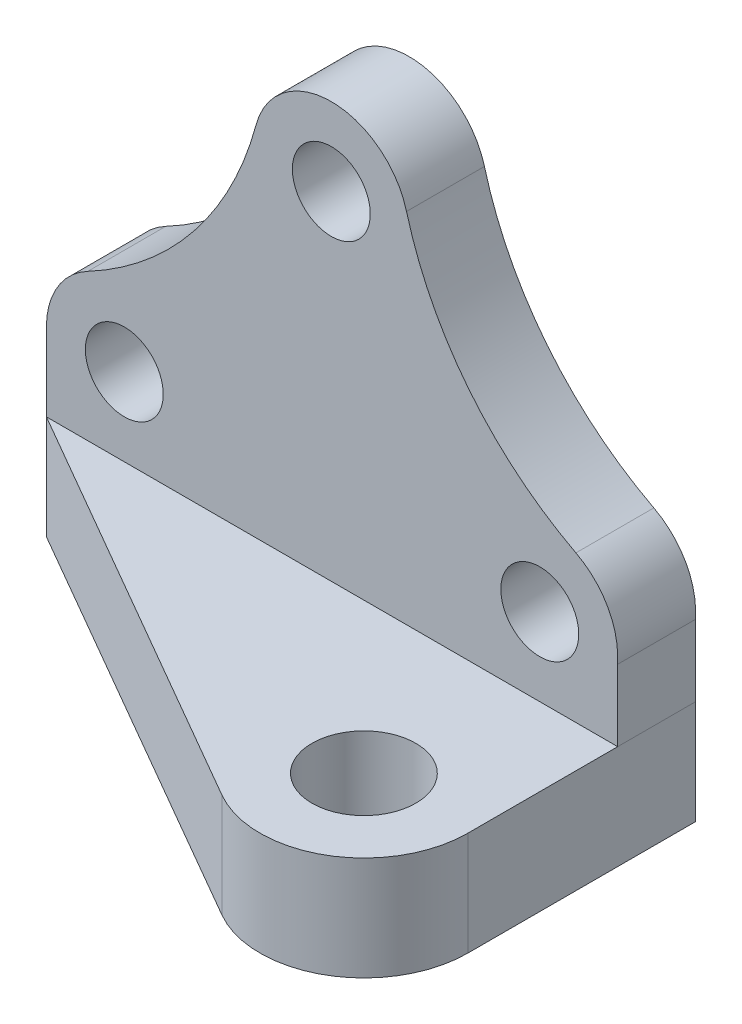
ISO-10303-21;
HEADER;
FILE_DESCRIPTION(('STEP AP214'),'2;1');
FILE_NAME('part.step','',(''),(''),'','','');
FILE_SCHEMA(('AUTOMOTIVE_DESIGN { 1 0 10303 214 1 1 1 1 }'));
ENDSEC;
DATA;
#1=APPLICATION_CONTEXT('core data for automotive mechanical design processes');
#2=APPLICATION_PROTOCOL_DEFINITION('international standard','automotive_design',2000,#1);
#3=PRODUCT_CONTEXT('',#1,'mechanical');
#4=PRODUCT('Part','Part','',(#3));
#5=PRODUCT_RELATED_PRODUCT_CATEGORY('part','',(#4));
#6=PRODUCT_DEFINITION_FORMATION('','',#4);
#7=PRODUCT_DEFINITION_CONTEXT('part definition',#1,'design');
#8=PRODUCT_DEFINITION('design','',#6,#7);
#9=PRODUCT_DEFINITION_SHAPE('','',#8);
#10=(LENGTH_UNIT() NAMED_UNIT(*) SI_UNIT(.MILLI.,.METRE.));
#11=(NAMED_UNIT(*) PLANE_ANGLE_UNIT() SI_UNIT($,.RADIAN.));
#12=(NAMED_UNIT(*) SI_UNIT($,.STERADIAN.) SOLID_ANGLE_UNIT());
#13=UNCERTAINTY_MEASURE_WITH_UNIT(LENGTH_MEASURE(1.E-05),#10,'distance_accuracy_value','');
#14=(GEOMETRIC_REPRESENTATION_CONTEXT(3) GLOBAL_UNCERTAINTY_ASSIGNED_CONTEXT((#13)) GLOBAL_UNIT_ASSIGNED_CONTEXT((#10,
#11,#12)) REPRESENTATION_CONTEXT('',''));
#15=CARTESIAN_POINT('',(0.,0.,0.));
#16=DIRECTION('',(0.,0.,1.));
#17=DIRECTION('',(1.,0.,0.));
#18=AXIS2_PLACEMENT_3D('',#15,#16,#17);
#19=CARTESIAN_POINT('',(0.,-20.,0.));
#20=DIRECTION('',(-0.500000000000001,0.,0.866025403784438));
#21=DIRECTION('',(0.866025403784438,0.,0.500000000000001));
#22=AXIS2_PLACEMENT_3D('',#19,#20,#21);
#23=PLANE('',#22);
#24=DIRECTION('',(0.866025403784438,0.,0.500000000000001));
#25=VECTOR('',#24,1.);
#26=CARTESIAN_POINT('',(0.,0.,0.));
#27=LINE('',#26,#25);
#28=CARTESIAN_POINT('',(0.,0.,0.));
#29=VERTEX_POINT('',#28);
#30=CARTESIAN_POINT('',(80.,0.,46.1880215351702));
#31=VERTEX_POINT('',#30);
#32=EDGE_CURVE('E102',#29,#31,#27,.T.);
#33=ORIENTED_EDGE('',*,*,#32,.F.);
#34=DIRECTION('',(0.,1.,0.));
#35=VECTOR('',#34,1.);
#36=CARTESIAN_POINT('',(0.,-20.,0.));
#37=LINE('',#36,#35);
#38=CARTESIAN_POINT('',(0.,-20.,0.));
#39=VERTEX_POINT('',#38);
#40=EDGE_CURVE('E11',#39,#29,#37,.T.);
#41=ORIENTED_EDGE('',*,*,#40,.F.);
#42=DIRECTION('',(0.866025403784438,0.,0.500000000000001));
#43=VECTOR('',#42,1.);
#44=CARTESIAN_POINT('',(0.,-20.,0.));
#45=LINE('',#44,#43);
#46=CARTESIAN_POINT('',(80.,-20.,46.1880215351702));
#47=VERTEX_POINT('',#46);
#48=EDGE_CURVE('E114',#39,#47,#45,.T.);
#49=ORIENTED_EDGE('',*,*,#48,.T.);
#50=DIRECTION('',(0.,1.,0.));
#51=VECTOR('',#50,1.);
#52=CARTESIAN_POINT('',(80.,-20.,46.1880215351702));
#53=LINE('',#52,#51);
#54=EDGE_CURVE('E42',#47,#31,#53,.T.);
#55=ORIENTED_EDGE('',*,*,#54,.T.);
#56=EDGE_LOOP('',(#33,#41,#49,#55));
#57=FACE_BOUND('',#56,.T.);
#58=ADVANCED_FACE('F41',(#57),#23,.T.);
#59=CARTESIAN_POINT('',(110.,-20.,0.));
#60=DIRECTION('',(1.,0.,0.));
#61=DIRECTION('',(0.,0.,-1.));
#62=AXIS2_PLACEMENT_3D('',#59,#60,#61);
#63=PLANE('',#62);
#64=DIRECTION('',(0.,0.,-1.));
#65=VECTOR('',#64,1.);
#66=CARTESIAN_POINT('',(110.,0.,0.));
#67=LINE('',#66,#65);
#68=CARTESIAN_POINT('',(110.,0.,28.8675134594814));
#69=VERTEX_POINT('',#68);
#70=CARTESIAN_POINT('',(110.,0.,0.));
#71=VERTEX_POINT('',#70);
#72=EDGE_CURVE('E115',#69,#71,#67,.T.);
#73=ORIENTED_EDGE('',*,*,#72,.F.);
#74=DIRECTION('',(0.,1.,0.));
#75=VECTOR('',#74,1.);
#76=CARTESIAN_POINT('',(110.,-20.,28.8675134594814));
#77=LINE('',#76,#75);
#78=CARTESIAN_POINT('',(110.,-20.,28.8675134594814));
#79=VERTEX_POINT('',#78);
#80=EDGE_CURVE('E49',#79,#69,#77,.T.);
#81=ORIENTED_EDGE('',*,*,#80,.F.);
#82=DIRECTION('',(0.,0.,-1.));
#83=VECTOR('',#82,1.);
#84=CARTESIAN_POINT('',(110.,-20.,0.));
#85=LINE('',#84,#83);
#86=CARTESIAN_POINT('',(110.,-20.,-15.));
#87=VERTEX_POINT('',#86);
#88=EDGE_CURVE('E118',#79,#87,#85,.T.);
#89=ORIENTED_EDGE('',*,*,#88,.T.);
#90=DIRECTION('',(0.,-1.,0.));
#91=VECTOR('',#90,1.);
#92=CARTESIAN_POINT('',(110.,0.,-15.));
#93=LINE('',#92,#91);
#94=CARTESIAN_POINT('',(110.,0.,-15.));
#95=VERTEX_POINT('',#94);
#96=EDGE_CURVE('E138',#95,#87,#93,.T.);
#97=ORIENTED_EDGE('',*,*,#96,.F.);
#98=DIRECTION('',(0.,0.,1.));
#99=VECTOR('',#98,1.);
#100=CARTESIAN_POINT('',(110.,0.,-15.));
#101=LINE('',#100,#99);
#102=EDGE_CURVE('E186',#95,#71,#101,.T.);
#103=ORIENTED_EDGE('',*,*,#102,.T.);
#104=EDGE_LOOP('',(#73,#81,#89,#97,#103));
#105=FACE_BOUND('',#104,.T.);
#106=ADVANCED_FACE('F224',(#105),#63,.T.);
#107=CARTESIAN_POINT('',(90.,-20.,28.8675134594814));
#108=DIRECTION('',(0.,1.,0.));
#109=DIRECTION('',(0.,0.,1.));
#110=AXIS2_PLACEMENT_3D('',#107,#108,#109);
#111=CYLINDRICAL_SURFACE('',#110,20.);
#112=CARTESIAN_POINT('',(90.,0.,28.8675134594814));
#113=DIRECTION('',(0.,1.,0.));
#114=DIRECTION('',(0.,0.,1.));
#115=AXIS2_PLACEMENT_3D('',#112,#113,#114);
#116=CIRCLE('',#115,20.);
#117=EDGE_CURVE('E110',#31,#69,#116,.T.);
#118=ORIENTED_EDGE('',*,*,#117,.F.);
#119=ORIENTED_EDGE('',*,*,#54,.F.);
#120=CARTESIAN_POINT('',(90.,-20.,28.8675134594814));
#121=DIRECTION('',(0.,1.,0.));
#122=DIRECTION('',(0.,0.,1.));
#123=AXIS2_PLACEMENT_3D('',#120,#121,#122);
#124=CIRCLE('',#123,20.);
#125=EDGE_CURVE('E113',#47,#79,#124,.T.);
#126=ORIENTED_EDGE('',*,*,#125,.T.);
#127=ORIENTED_EDGE('',*,*,#80,.T.);
#128=EDGE_LOOP('',(#118,#119,#126,#127));
#129=FACE_BOUND('',#128,.T.);
#130=ADVANCED_FACE('F124',(#129),#111,.T.);
#131=CARTESIAN_POINT('',(90.,-20.,28.8675134594814));
#132=DIRECTION('',(0.,1.,0.));
#133=DIRECTION('',(0.,0.,1.));
#134=AXIS2_PLACEMENT_3D('',#131,#132,#133);
#135=PLANE('',#134);
#136=CARTESIAN_POINT('',(90.,-20.,28.8675134594814));
#137=DIRECTION('',(0.,1.,0.));
#138=DIRECTION('',(0.,0.,1.));
#139=AXIS2_PLACEMENT_3D('',#136,#137,#138);
#140=CIRCLE('',#139,9.99999999999999);
#141=CARTESIAN_POINT('',(90.,-20.,38.8675134594814));
#142=VERTEX_POINT('',#141);
#143=EDGE_CURVE('E107',#142,#142,#140,.T.);
#144=ORIENTED_EDGE('',*,*,#143,.T.);
#145=EDGE_LOOP('',(#144));
#146=FACE_BOUND('',#145,.T.);
#147=ORIENTED_EDGE('',*,*,#48,.F.);
#148=DIRECTION('',(0.,0.,1.));
#149=VECTOR('',#148,1.);
#150=CARTESIAN_POINT('',(0.,-20.,-15.));
#151=LINE('',#150,#149);
#152=CARTESIAN_POINT('',(0.,-20.,-15.));
#153=VERTEX_POINT('',#152);
#154=EDGE_CURVE('E97',#153,#39,#151,.T.);
#155=ORIENTED_EDGE('',*,*,#154,.F.);
#156=DIRECTION('',(-1.,0.,0.));
#157=VECTOR('',#156,1.);
#158=CARTESIAN_POINT('',(0.,-20.,-15.));
#159=LINE('',#158,#157);
#160=EDGE_CURVE('E134',#87,#153,#159,.T.);
#161=ORIENTED_EDGE('',*,*,#160,.F.);
#162=ORIENTED_EDGE('',*,*,#88,.F.);
#163=ORIENTED_EDGE('',*,*,#125,.F.);
#164=EDGE_LOOP('',(#147,#155,#161,#162,#163));
#165=FACE_BOUND('',#164,.T.);
#166=ADVANCED_FACE('F126',(#146,#165),#135,.F.);
#167=CARTESIAN_POINT('',(90.,0.,28.8675134594814));
#168=DIRECTION('',(0.,1.,0.));
#169=DIRECTION('',(0.,0.,1.));
#170=AXIS2_PLACEMENT_3D('',#167,#168,#169);
#171=PLANE('',#170);
#172=CARTESIAN_POINT('',(90.,0.,28.8675134594814));
#173=DIRECTION('',(0.,1.,0.));
#174=DIRECTION('',(0.,0.,1.));
#175=AXIS2_PLACEMENT_3D('',#172,#173,#174);
#176=CIRCLE('',#175,9.99999999999999);
#177=CARTESIAN_POINT('',(90.,0.,38.8675134594814));
#178=VERTEX_POINT('',#177);
#179=EDGE_CURVE('E203',#178,#178,#176,.T.);
#180=ORIENTED_EDGE('',*,*,#179,.F.);
#181=EDGE_LOOP('',(#180));
#182=FACE_BOUND('',#181,.T.);
#183=ORIENTED_EDGE('',*,*,#32,.T.);
#184=ORIENTED_EDGE('',*,*,#117,.T.);
#185=ORIENTED_EDGE('',*,*,#72,.T.);
#186=DIRECTION('',(-1.,0.,0.));
#187=VECTOR('',#186,1.);
#188=CARTESIAN_POINT('',(0.,0.,0.));
#189=LINE('',#188,#187);
#190=EDGE_CURVE('E85',#71,#29,#189,.T.);
#191=ORIENTED_EDGE('',*,*,#190,.T.);
#192=EDGE_LOOP('',(#183,#184,#185,#191));
#193=FACE_BOUND('',#192,.T.);
#194=ADVANCED_FACE('F112',(#182,#193),#171,.T.);
#195=CARTESIAN_POINT('',(90.,-20.,28.8675134594814));
#196=DIRECTION('',(0.,1.,0.));
#197=DIRECTION('',(0.,0.,1.));
#198=AXIS2_PLACEMENT_3D('',#195,#196,#197);
#199=CYLINDRICAL_SURFACE('',#198,9.99999999999999);
#200=ORIENTED_EDGE('',*,*,#143,.F.);
#201=EDGE_LOOP('',(#200));
#202=FACE_BOUND('',#201,.T.);
#203=ORIENTED_EDGE('',*,*,#179,.T.);
#204=EDGE_LOOP('',(#203));
#205=FACE_BOUND('',#204,.T.);
#206=ADVANCED_FACE('F210',(#202,#205),#199,.F.);
#207=CARTESIAN_POINT('',(-22.4100448127981,85.7141325839781,-15.));
#208=DIRECTION('',(0.,0.,1.));
#209=DIRECTION('',(1.,0.,0.));
#210=AXIS2_PLACEMENT_3D('',#207,#208,#209);
#211=CYLINDRICAL_SURFACE('',#210,65.);
#212=CARTESIAN_POINT('',(-22.4100448127981,85.7141325839781,0.));
#213=DIRECTION('',(0.,0.,-1.));
#214=DIRECTION('',(-1.,0.,0.));
#215=AXIS2_PLACEMENT_3D('',#212,#213,#214);
#216=CIRCLE('',#215,65.);
#217=CARTESIAN_POINT('',(40.3732592292779,68.8838998594959,0.));
#218=VERTEX_POINT('',#217);
#219=CARTESIAN_POINT('',(7.98561659760035,28.2588998594959,0.));
#220=VERTEX_POINT('',#219);
#221=EDGE_CURVE('E158',#218,#220,#216,.T.);
#222=ORIENTED_EDGE('',*,*,#221,.F.);
#223=DIRECTION('',(0.,0.,1.));
#224=VECTOR('',#223,1.);
#225=CARTESIAN_POINT('',(40.3732592292779,68.8838998594959,-15.));
#226=LINE('',#225,#224);
#227=CARTESIAN_POINT('',(40.3732592292779,68.8838998594959,-15.));
#228=VERTEX_POINT('',#227);
#229=EDGE_CURVE('E196',#228,#218,#226,.T.);
#230=ORIENTED_EDGE('',*,*,#229,.F.);
#231=CARTESIAN_POINT('',(-22.4100448127981,85.7141325839781,-15.));
#232=DIRECTION('',(0.,0.,-1.));
#233=DIRECTION('',(-1.,0.,0.));
#234=AXIS2_PLACEMENT_3D('',#231,#232,#233);
#235=CIRCLE('',#234,65.);
#236=CARTESIAN_POINT('',(7.98561659760035,28.2588998594959,-15.));
#237=VERTEX_POINT('',#236);
#238=EDGE_CURVE('E179',#228,#237,#235,.T.);
#239=ORIENTED_EDGE('',*,*,#238,.T.);
#240=DIRECTION('',(0.,0.,1.));
#241=VECTOR('',#240,1.);
#242=CARTESIAN_POINT('',(7.98561659760035,28.2588998594959,-15.));
#243=LINE('',#242,#241);
#244=EDGE_CURVE('E160',#237,#220,#243,.T.);
#245=ORIENTED_EDGE('',*,*,#244,.T.);
#246=EDGE_LOOP('',(#222,#230,#239,#245));
#247=FACE_BOUND('',#246,.T.);
#248=ADVANCED_FACE('F216',(#247),#211,.F.);
#249=CARTESIAN_POINT('',(54.8617140082186,65.,-15.));
#250=DIRECTION('',(0.,0.,1.));
#251=DIRECTION('',(1.,0.,0.));
#252=AXIS2_PLACEMENT_3D('',#249,#250,#251);
#253=CYLINDRICAL_SURFACE('',#252,15.);
#254=CARTESIAN_POINT('',(54.8617140082186,65.,0.));
#255=DIRECTION('',(0.,0.,-1.));
#256=DIRECTION('',(-1.,0.,0.));
#257=AXIS2_PLACEMENT_3D('',#254,#255,#256);
#258=CIRCLE('',#257,15.);
#259=CARTESIAN_POINT('',(69.3416105706828,68.9156858326908,0.));
#260=VERTEX_POINT('',#259);
#261=EDGE_CURVE('E159',#218,#260,#258,.T.);
#262=ORIENTED_EDGE('',*,*,#261,.T.);
#263=DIRECTION('',(0.,0.,1.));
#264=VECTOR('',#263,1.);
#265=CARTESIAN_POINT('',(69.3416105706828,68.9156858326908,-15.));
#266=LINE('',#265,#264);
#267=CARTESIAN_POINT('',(69.3416105706828,68.9156858326908,-15.));
#268=VERTEX_POINT('',#267);
#269=EDGE_CURVE('E194',#268,#260,#266,.T.);
#270=ORIENTED_EDGE('',*,*,#269,.F.);
#271=CARTESIAN_POINT('',(54.8617140082186,65.,-15.));
#272=DIRECTION('',(0.,0.,-1.));
#273=DIRECTION('',(-1.,0.,0.));
#274=AXIS2_PLACEMENT_3D('',#271,#272,#273);
#275=CIRCLE('',#274,15.);
#276=EDGE_CURVE('E333',#228,#268,#275,.T.);
#277=ORIENTED_EDGE('',*,*,#276,.F.);
#278=ORIENTED_EDGE('',*,*,#229,.T.);
#279=EDGE_LOOP('',(#262,#270,#277,#278));
#280=FACE_BOUND('',#279,.T.);
#281=ADVANCED_FACE('F284',(#280),#253,.T.);
#282=CARTESIAN_POINT('',(132.087829008028,85.8836577743507,-15.));
#283=DIRECTION('',(0.,0.,1.));
#284=DIRECTION('',(1.,0.,0.));
#285=AXIS2_PLACEMENT_3D('',#282,#283,#284);
#286=CYLINDRICAL_SURFACE('',#285,65.);
#287=CARTESIAN_POINT('',(132.087829008028,85.8836577743507,0.));
#288=DIRECTION('',(0.,0.,-1.));
#289=DIRECTION('',(-1.,0.,0.));
#290=AXIS2_PLACEMENT_3D('',#287,#288,#289);
#291=CIRCLE('',#290,65.);
#292=CARTESIAN_POINT('',(101.953967939005,28.2906858326908,0.));
#293=VERTEX_POINT('',#292);
#294=EDGE_CURVE('E162',#293,#260,#291,.T.);
#295=ORIENTED_EDGE('',*,*,#294,.F.);
#296=DIRECTION('',(0.,0.,1.));
#297=VECTOR('',#296,1.);
#298=CARTESIAN_POINT('',(101.953967939005,28.2906858326908,-15.));
#299=LINE('',#298,#297);
#300=CARTESIAN_POINT('',(101.953967939005,28.2906858326908,-15.));
#301=VERTEX_POINT('',#300);
#302=EDGE_CURVE('E195',#301,#293,#299,.T.);
#303=ORIENTED_EDGE('',*,*,#302,.F.);
#304=CARTESIAN_POINT('',(132.087829008028,85.8836577743507,-15.));
#305=DIRECTION('',(0.,0.,-1.));
#306=DIRECTION('',(-1.,0.,0.));
#307=AXIS2_PLACEMENT_3D('',#304,#305,#306);
#308=CIRCLE('',#307,65.);
#309=EDGE_CURVE('E279',#301,#268,#308,.T.);
#310=ORIENTED_EDGE('',*,*,#309,.T.);
#311=ORIENTED_EDGE('',*,*,#269,.T.);
#312=EDGE_LOOP('',(#295,#303,#310,#311));
#313=FACE_BOUND('',#312,.T.);
#314=ADVANCED_FACE('F277',(#313),#286,.F.);
#315=CARTESIAN_POINT('',(95.,15.,-15.));
#316=DIRECTION('',(0.,0.,1.));
#317=DIRECTION('',(1.,0.,0.));
#318=AXIS2_PLACEMENT_3D('',#315,#316,#317);
#319=CYLINDRICAL_SURFACE('',#318,15.);
#320=CARTESIAN_POINT('',(95.,15.,0.));
#321=DIRECTION('',(0.,0.,-1.));
#322=DIRECTION('',(-1.,0.,0.));
#323=AXIS2_PLACEMENT_3D('',#320,#321,#322);
#324=CIRCLE('',#323,15.);
#325=CARTESIAN_POINT('',(109.941701745293,13.6788077525573,0.));
#326=VERTEX_POINT('',#325);
#327=EDGE_CURVE('E167',#293,#326,#324,.T.);
#328=ORIENTED_EDGE('',*,*,#327,.T.);
#329=DIRECTION('',(0.,0.,1.));
#330=VECTOR('',#329,1.);
#331=CARTESIAN_POINT('',(109.941701745293,13.6788077525573,-15.));
#332=LINE('',#331,#330);
#333=CARTESIAN_POINT('',(109.941701745293,13.6788077525573,-15.));
#334=VERTEX_POINT('',#333);
#335=EDGE_CURVE('E188',#334,#326,#332,.T.);
#336=ORIENTED_EDGE('',*,*,#335,.F.);
#337=CARTESIAN_POINT('',(95.,15.,-15.));
#338=DIRECTION('',(0.,0.,-1.));
#339=DIRECTION('',(-1.,0.,0.));
#340=AXIS2_PLACEMENT_3D('',#337,#338,#339);
#341=CIRCLE('',#340,15.);
#342=EDGE_CURVE('E341',#301,#334,#341,.T.);
#343=ORIENTED_EDGE('',*,*,#342,.F.);
#344=ORIENTED_EDGE('',*,*,#302,.T.);
#345=EDGE_LOOP('',(#328,#336,#343,#344));
#346=FACE_BOUND('',#345,.T.);
#347=ADVANCED_FACE('F289',(#346),#319,.T.);
#348=CARTESIAN_POINT('',(109.99800198193,0.468804858784846,-15.));
#349=DIRECTION('',(0.999990918058441,0.00426190105892585,0.));
#350=DIRECTION('',(-0.00426190105892585,0.999990918058441,0.));
#351=AXIS2_PLACEMENT_3D('',#348,#349,#350);
#352=PLANE('',#351);
#353=DIRECTION('',(-0.00426190105892585,0.999990918058441,0.));
#354=VECTOR('',#353,1.);
#355=CARTESIAN_POINT('',(109.99800198193,0.468804858784846,0.));
#356=LINE('',#355,#354);
#357=EDGE_CURVE('E89',#71,#326,#356,.T.);
#358=ORIENTED_EDGE('',*,*,#357,.F.);
#359=ORIENTED_EDGE('',*,*,#102,.F.);
#360=DIRECTION('',(-0.00426190105892585,0.999990918058441,0.));
#361=VECTOR('',#360,1.);
#362=CARTESIAN_POINT('',(109.99800198193,0.468804858784846,-15.));
#363=LINE('',#362,#361);
#364=EDGE_CURVE('E142',#95,#334,#363,.T.);
#365=ORIENTED_EDGE('',*,*,#364,.T.);
#366=ORIENTED_EDGE('',*,*,#335,.T.);
#367=EDGE_LOOP('',(#358,#359,#365,#366));
#368=FACE_BOUND('',#367,.T.);
#369=ADVANCED_FACE('F240',(#368),#352,.T.);
#370=CARTESIAN_POINT('',(0.,0.,-15.));
#371=DIRECTION('',(-1.,0.,0.));
#372=DIRECTION('',(0.,0.,1.));
#373=AXIS2_PLACEMENT_3D('',#370,#371,#372);
#374=PLANE('',#373);
#375=DIRECTION('',(0.,-1.,0.));
#376=VECTOR('',#375,1.);
#377=CARTESIAN_POINT('',(0.,0.,0.));
#378=LINE('',#377,#376);
#379=CARTESIAN_POINT('',(0.,15.,0.));
#380=VERTEX_POINT('',#379);
#381=EDGE_CURVE('E79',#380,#29,#378,.T.);
#382=ORIENTED_EDGE('',*,*,#381,.F.);
#383=DIRECTION('',(0.,0.,1.));
#384=VECTOR('',#383,1.);
#385=CARTESIAN_POINT('',(0.,15.,-15.));
#386=LINE('',#385,#384);
#387=CARTESIAN_POINT('',(0.,15.,-15.));
#388=VERTEX_POINT('',#387);
#389=EDGE_CURVE('E181',#388,#380,#386,.T.);
#390=ORIENTED_EDGE('',*,*,#389,.F.);
#391=DIRECTION('',(0.,-1.,0.));
#392=VECTOR('',#391,1.);
#393=CARTESIAN_POINT('',(0.,0.,-15.));
#394=LINE('',#393,#392);
#395=EDGE_CURVE('E140',#388,#153,#394,.T.);
#396=ORIENTED_EDGE('',*,*,#395,.T.);
#397=ORIENTED_EDGE('',*,*,#154,.T.);
#398=ORIENTED_EDGE('',*,*,#40,.T.);
#399=EDGE_LOOP('',(#382,#390,#396,#397,#398));
#400=FACE_BOUND('',#399,.T.);
#401=ADVANCED_FACE('F92',(#400),#374,.T.);
#402=CARTESIAN_POINT('',(15.,15.,-15.));
#403=DIRECTION('',(0.,0.,1.));
#404=DIRECTION('',(1.,0.,0.));
#405=AXIS2_PLACEMENT_3D('',#402,#403,#404);
#406=CYLINDRICAL_SURFACE('',#405,7.5);
#407=CARTESIAN_POINT('',(15.,15.,-15.));
#408=DIRECTION('',(0.,0.,-1.));
#409=DIRECTION('',(-1.,0.,0.));
#410=AXIS2_PLACEMENT_3D('',#407,#408,#409);
#411=CIRCLE('',#410,7.5);
#412=CARTESIAN_POINT('',(7.5,15.,-15.));
#413=VERTEX_POINT('',#412);
#414=EDGE_CURVE('E151',#413,#413,#411,.T.);
#415=ORIENTED_EDGE('',*,*,#414,.T.);
#416=EDGE_LOOP('',(#415));
#417=FACE_BOUND('',#416,.T.);
#418=CARTESIAN_POINT('',(15.,15.,0.));
#419=DIRECTION('',(0.,0.,-1.));
#420=DIRECTION('',(-1.,0.,0.));
#421=AXIS2_PLACEMENT_3D('',#418,#419,#420);
#422=CIRCLE('',#421,7.5);
#423=CARTESIAN_POINT('',(7.5,15.,0.));
#424=VERTEX_POINT('',#423);
#425=EDGE_CURVE('E173',#424,#424,#422,.T.);
#426=ORIENTED_EDGE('',*,*,#425,.F.);
#427=EDGE_LOOP('',(#426));
#428=FACE_BOUND('',#427,.T.);
#429=ADVANCED_FACE('F300',(#417,#428),#406,.F.);
#430=CARTESIAN_POINT('',(54.8617140082186,65.,-15.));
#431=DIRECTION('',(0.,0.,1.));
#432=DIRECTION('',(1.,0.,0.));
#433=AXIS2_PLACEMENT_3D('',#430,#431,#432);
#434=CYLINDRICAL_SURFACE('',#433,7.5);
#435=CARTESIAN_POINT('',(54.8617140082186,65.,-15.));
#436=DIRECTION('',(0.,0.,-1.));
#437=DIRECTION('',(-1.,0.,0.));
#438=AXIS2_PLACEMENT_3D('',#435,#436,#437);
#439=CIRCLE('',#438,7.5);
#440=CARTESIAN_POINT('',(47.3617140082186,65.,-15.));
#441=VERTEX_POINT('',#440);
#442=EDGE_CURVE('E146',#441,#441,#439,.T.);
#443=ORIENTED_EDGE('',*,*,#442,.T.);
#444=EDGE_LOOP('',(#443));
#445=FACE_BOUND('',#444,.T.);
#446=CARTESIAN_POINT('',(54.8617140082186,65.,0.));
#447=DIRECTION('',(0.,0.,-1.));
#448=DIRECTION('',(-1.,0.,0.));
#449=AXIS2_PLACEMENT_3D('',#446,#447,#448);
#450=CIRCLE('',#449,7.5);
#451=CARTESIAN_POINT('',(47.3617140082186,65.,0.));
#452=VERTEX_POINT('',#451);
#453=EDGE_CURVE('E174',#452,#452,#450,.T.);
#454=ORIENTED_EDGE('',*,*,#453,.F.);
#455=EDGE_LOOP('',(#454));
#456=FACE_BOUND('',#455,.T.);
#457=ADVANCED_FACE('F303',(#445,#456),#434,.F.);
#458=CARTESIAN_POINT('',(15.,15.,-15.));
#459=DIRECTION('',(0.,0.,1.));
#460=DIRECTION('',(1.,0.,0.));
#461=AXIS2_PLACEMENT_3D('',#458,#459,#460);
#462=CYLINDRICAL_SURFACE('',#461,15.);
#463=CARTESIAN_POINT('',(15.,15.,0.));
#464=DIRECTION('',(0.,0.,-1.));
#465=DIRECTION('',(-1.,0.,0.));
#466=AXIS2_PLACEMENT_3D('',#463,#464,#465);
#467=CIRCLE('',#466,15.);
#468=EDGE_CURVE('E87',#380,#220,#467,.T.);
#469=ORIENTED_EDGE('',*,*,#468,.T.);
#470=ORIENTED_EDGE('',*,*,#244,.F.);
#471=CARTESIAN_POINT('',(15.,15.,-15.));
#472=DIRECTION('',(0.,0.,-1.));
#473=DIRECTION('',(-1.,0.,0.));
#474=AXIS2_PLACEMENT_3D('',#471,#472,#473);
#475=CIRCLE('',#474,15.);
#476=EDGE_CURVE('E139',#388,#237,#475,.T.);
#477=ORIENTED_EDGE('',*,*,#476,.F.);
#478=ORIENTED_EDGE('',*,*,#389,.T.);
#479=EDGE_LOOP('',(#469,#470,#477,#478));
#480=FACE_BOUND('',#479,.T.);
#481=ADVANCED_FACE('F298',(#480),#462,.T.);
#482=CARTESIAN_POINT('',(95.,15.,-15.));
#483=DIRECTION('',(0.,0.,1.));
#484=DIRECTION('',(1.,0.,0.));
#485=AXIS2_PLACEMENT_3D('',#482,#483,#484);
#486=CYLINDRICAL_SURFACE('',#485,7.50000000000001);
#487=CARTESIAN_POINT('',(95.,15.,-15.));
#488=DIRECTION('',(0.,0.,-1.));
#489=DIRECTION('',(-1.,0.,0.));
#490=AXIS2_PLACEMENT_3D('',#487,#488,#489);
#491=CIRCLE('',#490,7.50000000000001);
#492=CARTESIAN_POINT('',(87.5,15.,-15.));
#493=VERTEX_POINT('',#492);
#494=EDGE_CURVE('E152',#493,#493,#491,.T.);
#495=ORIENTED_EDGE('',*,*,#494,.T.);
#496=EDGE_LOOP('',(#495));
#497=FACE_BOUND('',#496,.T.);
#498=CARTESIAN_POINT('',(95.,15.,0.));
#499=DIRECTION('',(0.,0.,-1.));
#500=DIRECTION('',(-1.,0.,0.));
#501=AXIS2_PLACEMENT_3D('',#498,#499,#500);
#502=CIRCLE('',#501,7.50000000000001);
#503=CARTESIAN_POINT('',(87.5,15.,0.));
#504=VERTEX_POINT('',#503);
#505=EDGE_CURVE('E180',#504,#504,#502,.T.);
#506=ORIENTED_EDGE('',*,*,#505,.F.);
#507=EDGE_LOOP('',(#506));
#508=FACE_BOUND('',#507,.T.);
#509=ADVANCED_FACE('F305',(#497,#508),#486,.F.);
#510=CARTESIAN_POINT('',(0.,0.,-15.));
#511=DIRECTION('',(0.,0.,-1.));
#512=DIRECTION('',(-1.,0.,0.));
#513=AXIS2_PLACEMENT_3D('',#510,#511,#512);
#514=PLANE('',#513);
#515=ORIENTED_EDGE('',*,*,#238,.F.);
#516=ORIENTED_EDGE('',*,*,#276,.T.);
#517=ORIENTED_EDGE('',*,*,#309,.F.);
#518=ORIENTED_EDGE('',*,*,#342,.T.);
#519=ORIENTED_EDGE('',*,*,#364,.F.);
#520=ORIENTED_EDGE('',*,*,#96,.T.);
#521=ORIENTED_EDGE('',*,*,#160,.T.);
#522=ORIENTED_EDGE('',*,*,#395,.F.);
#523=ORIENTED_EDGE('',*,*,#476,.T.);
#524=EDGE_LOOP('',(#515,#516,#517,#518,#519,#520,#521,#522,#523));
#525=FACE_BOUND('',#524,.T.);
#526=ORIENTED_EDGE('',*,*,#442,.F.);
#527=EDGE_LOOP('',(#526));
#528=FACE_BOUND('',#527,.T.);
#529=ORIENTED_EDGE('',*,*,#414,.F.);
#530=EDGE_LOOP('',(#529));
#531=FACE_BOUND('',#530,.T.);
#532=ORIENTED_EDGE('',*,*,#494,.F.);
#533=EDGE_LOOP('',(#532));
#534=FACE_BOUND('',#533,.T.);
#535=ADVANCED_FACE('F311',(#525,#528,#531,#534),#514,.T.);
#536=CARTESIAN_POINT('',(0.,0.,0.));
#537=DIRECTION('',(0.,0.,-1.));
#538=DIRECTION('',(-1.,0.,0.));
#539=AXIS2_PLACEMENT_3D('',#536,#537,#538);
#540=PLANE('',#539);
#541=ORIENTED_EDGE('',*,*,#190,.F.);
#542=ORIENTED_EDGE('',*,*,#357,.T.);
#543=ORIENTED_EDGE('',*,*,#327,.F.);
#544=ORIENTED_EDGE('',*,*,#294,.T.);
#545=ORIENTED_EDGE('',*,*,#261,.F.);
#546=ORIENTED_EDGE('',*,*,#221,.T.);
#547=ORIENTED_EDGE('',*,*,#468,.F.);
#548=ORIENTED_EDGE('',*,*,#381,.T.);
#549=EDGE_LOOP('',(#541,#542,#543,#544,#545,#546,#547,#548));
#550=FACE_BOUND('',#549,.T.);
#551=ORIENTED_EDGE('',*,*,#453,.T.);
#552=EDGE_LOOP('',(#551));
#553=FACE_BOUND('',#552,.T.);
#554=ORIENTED_EDGE('',*,*,#425,.T.);
#555=EDGE_LOOP('',(#554));
#556=FACE_BOUND('',#555,.T.);
#557=ORIENTED_EDGE('',*,*,#505,.T.);
#558=EDGE_LOOP('',(#557));
#559=FACE_BOUND('',#558,.T.);
#560=ADVANCED_FACE('F76',(#550,#553,#556,#559),#540,.F.);
#561=CLOSED_SHELL('',(#58,#106,#130,#166,#194,#206,#248,#281,#314,#347,#369,#401,#429,#457,#481,
#509,#535,#560));
#562=MANIFOLD_SOLID_BREP('B2',#561);
#563=ADVANCED_BREP_SHAPE_REPRESENTATION('',(#18,#562),#14);
#564=SHAPE_DEFINITION_REPRESENTATION(#9,#563);
ENDSEC;
END-ISO-10303-21;
